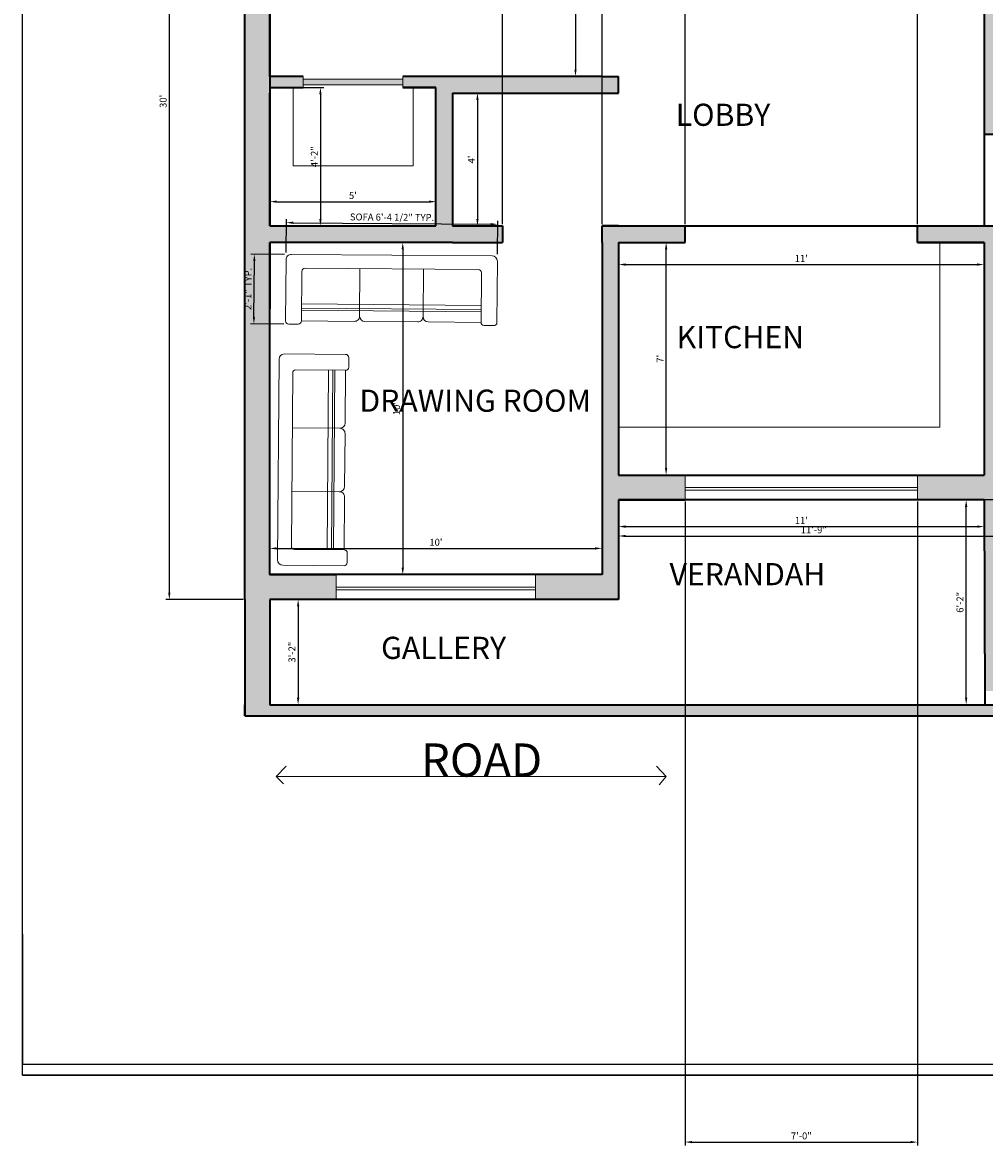
# Model space of a CAD drawing. Units: inches. Extents: x 2341 to 2872, y 1788 to 2419.
# Tile 1 of 3: x 2341 to 2689, y 1788 to 2194. Entities that reach past the tile are written whole.
import ezdxf

# ---------------------------------------------------------------- set-up
doc = ezdxf.new("R2010")
doc.units = ezdxf.units.IN
for name, color, linetype, lineweight in [('A-ANNO-DIMS', 2, 'Continuous', 18), ('A-ANNO-SYMB', 7, 'Continuous', 18), ('A-ANNO-TEXT', 7, 'Continuous', 25), ('A-ANNO-TTLB', 7, 'Continuous', 25), ('A-AREA-IDEN', 7, 'Continuous', 25), ('A-FLOR-FIXT', 9, 'Continuous', 18), ('A-FURN', 8, 'Continuous', 18), ('A-GLAZ', 4, 'Continuous', 18), ('A-WALL', 7, 'Continuous', 35)]:
    doc.layers.add(name, color=color, linetype=linetype, lineweight=lineweight)
doc.layers.add('A-WALL-PATT', color=18, linetype='Continuous', lineweight=13, true_color=0x000000)
doc.styles.get("Standard").update_dxf_attribs({"font": 'arial.ttf'})
doc.dimstyles.new('Copy of ISO-25', dxfattribs={"dimtxt": 2.5, "dimasz": 2.5, "dimexe": 1.25, "dimexo": 0.625, "dimtad": 1, "dimdec": 1, "dimlunit": 4, "dimtxsty": 'Standard', "dimcen": 2.5, "dimadec": 0, "dimazin": 0, "dimtfac": 1, "dimtdec": 1, "dimtmove": 0, "dimatfit": 3, "dimfxl": 1, "dimarcsym": 0})

# ---------------------------------------------------------------- blocks, each defined once
blk = doc.blocks.new('A$C05BA3A2B')
for p, q in [((0.05, 0.66), (1.95, 0.66)), ((0.05, 0.66), (1.95, 0.66)), ((0.05, 0.66), (1.95, 0.66)), ((0, 0.03), (0, 0.61)), ((0, 0.03), (0, 0.61)), ((0, 0.03), (0, 0.61)), ((2, 0.61), (2, 0.03)), ((2, 0.61), (2, 0.03)), ((2, 0.61), (2, 0.03)), ((0.15, 0.5), (0.15, 0.03)), ((0.15, 0.5), (0.15, 0.03)), ((0.15, 0.5), (0.15, 0.03)), ((1.82, 0.53), (0.18, 0.53)), ((1.82, 0.53), (0.18, 0.53)), ((1.82, 0.53), (0.18, 0.53)), ((0.7, 0.08), (0.7, 0.53)), ((0.7, 0.08), (0.7, 0.53)), ((0.7, 0.08), (0.7, 0.53)), ((1.3, 0.53), (1.3, 0.08)), ((1.3, 0.53), (1.3, 0.08)), ((1.3, 0.53), (1.3, 0.08)), ((1.85, 0.03), (1.85, 0.5)), ((1.85, 0.03), (1.85, 0.5)), ((1.85, 0.03), (1.85, 0.5)), ((1.85, 0.191), (0.15, 0.191)), ((1.85, 0.191), (0.15, 0.191)), ((1.85, 0.191), (0.15, 0.191)), ((1.85, 0.151), (0.15, 0.151)), ((1.85, 0.151), (0.15, 0.151)), ((1.85, 0.151), (0.15, 0.151)), ((1.85, 0.131), (0.15, 0.131)), ((1.85, 0.131), (0.15, 0.131)), ((1.85, 0.131), (0.15, 0.131)), ((0.12, 0), (0.03, 0)), ((0.12, 0), (0.03, 0)), ((0.12, 0), (0.03, 0)), ((0.65, 0.03), (0.15, 0.03)), ((0.65, 0.03), (0.15, 0.03)), ((0.65, 0.03), (0.15, 0.03)), ((1.25, 0.03), (0.75, 0.03)), ((1.25, 0.03), (0.75, 0.03)), ((1.25, 0.03), (0.75, 0.03)), ((1.85, 0.03), (1.35, 0.03)), ((1.85, 0.03), (1.35, 0.03)), ((1.85, 0.03), (1.35, 0.03)), ((1.97, 0), (1.88, 0)), ((1.97, 0), (1.88, 0)), ((1.97, 0), (1.88, 0))]:
    blk.add_line(p, q)
for centre, radius, start, end in [((0.05, 0.61), 0.05, 90, 180), ((0.05, 0.61), 0.05, 90, 180), ((0.05, 0.61), 0.05, 90, 180), ((1.95, 0.61), 0.05, 0, 90), ((1.95, 0.61), 0.05, 0, 90), ((1.95, 0.61), 0.05, 0, 90), ((0.18, 0.5), 0.03, 90, 180), ((0.18, 0.5), 0.03, 90, 180), ((0.18, 0.5), 0.03, 90, 180), ((1.82, 0.5), 0.03, 0, 90), ((1.82, 0.5), 0.03, 0, 90), ((1.82, 0.5), 0.03, 0, 90), ((0.03, 0.03), 0.03, 180, 270), ((0.03, 0.03), 0.03, 180, 270), ((0.03, 0.03), 0.03, 180, 270), ((0.12, 0.03), 0.03, 270, 0), ((0.12, 0.03), 0.03, 270, 0), ((0.12, 0.03), 0.03, 270, 0), ((0.65, 0.08), 0.05, 270, 0), ((0.65, 0.08), 0.05, 270, 0), ((0.65, 0.08), 0.05, 270, 0), ((0.75, 0.08), 0.05, 180, 270), ((0.75, 0.08), 0.05, 180, 270), ((0.75, 0.08), 0.05, 180, 270), ((1.25, 0.08), 0.05, 270, 0), ((1.25, 0.08), 0.05, 270, 0), ((1.25, 0.08), 0.05, 270, 0), ((1.35, 0.08), 0.05, 180, 270), ((1.35, 0.08), 0.05, 180, 270), ((1.35, 0.08), 0.05, 180, 270), ((1.88, 0.03), 0.03, 180, 270), ((1.88, 0.03), 0.03, 180, 270), ((1.88, 0.03), 0.03, 180, 270), ((1.97, 0.03), 0.03, 270, 0), ((1.97, 0.03), 0.03, 270, 0), ((1.97, 0.03), 0.03, 270, 0)]:
    blk.add_arc(centre, radius, start, end)
blk = doc.blocks.new('*D4')
at = {"layer": 'A-ANNO-DIMS', "color": 0, "lineweight": -2, "transparency": 16777216}
for p, q in [((2420.93, 2345.02), (2392.99, 2345.02)), ((2394.24, 2342.52), (2394.24, 1987.52)), ((2420.93, 1985.02), (2392.99, 1985.02))]:
    blk.add_line(p, q, dxfattribs=at)
at = {"layer": 'A-ANNO-DIMS', "color": 0, "transparency": 16777216}
for points in [[(2393.82, 2342.52), (2394.66, 2342.52), (2394.24, 2345.02)], [(2393.82, 1987.52), (2394.66, 1987.52), (2394.24, 1985.02)]]:
    blk.add_solid(points, dxfattribs=at)
at = {"layer": 'Defpoints', "color": 0, "transparency": 16777216}
for p in [(2421.55, 2345.02), (2394.24, 1985.02), (2421.55, 1985.02)]:
    blk.add_point(p, dxfattribs=at)
at = {"layer": 'A-ANNO-DIMS', "color": 0, "transparency": 16777216, "insert": (2392.34, 2165.02), "char_height": 2.5, "attachment_point": 5, "rotation": 90}
blk.add_mtext("30'", dxfattribs=at)
blk = doc.blocks.new('*D8')
at = {"layer": 'A-ANNO-DIMS', "color": 0, "lineweight": -2, "transparency": 16777216}
for p, q in [((2549.93, 2336.02), (2539.72, 2336.02)), ((2540.97, 2333.52), (2540.97, 2176.52)), ((2549.93, 2174.02), (2539.72, 2174.02))]:
    blk.add_line(p, q, dxfattribs=at)
at = {"layer": 'A-ANNO-DIMS', "color": 0, "transparency": 16777216}
for points in [[(2540.56, 2333.52), (2541.39, 2333.52), (2540.97, 2336.02)], [(2540.56, 2176.52), (2541.39, 2176.52), (2540.97, 2174.02)]]:
    blk.add_solid(points, dxfattribs=at)
at = {"layer": 'Defpoints', "color": 0, "transparency": 16777216}
for p in [(2550.55, 2336.02), (2540.97, 2174.02), (2550.55, 2174.02)]:
    blk.add_point(p, dxfattribs=at)
at = {"layer": 'A-ANNO-DIMS', "color": 0, "transparency": 16777216, "insert": (2539.07, 2255.02), "char_height": 2.5, "attachment_point": 5, "rotation": 90}
blk.add_mtext('13\'-6"', dxfattribs=at)
blk = doc.blocks.new('*D17')
at = {"layer": 'A-ANNO-DIMS', "color": 0, "lineweight": -2, "transparency": 16777216}
for p, q in [((2431.18, 2114.02), (2479.82, 2114.02)), ((2478.57, 2111.52), (2478.57, 1996.52)), ((2431.18, 1994.02), (2479.82, 1994.02))]:
    blk.add_line(p, q, dxfattribs=at)
at = {"layer": 'A-ANNO-DIMS', "color": 0, "transparency": 16777216}
for points in [[(2478.15, 2111.52), (2478.99, 2111.52), (2478.57, 2114.02)], [(2478.15, 1996.52), (2478.99, 1996.52), (2478.57, 1994.02)]]:
    blk.add_solid(points, dxfattribs=at)
at = {"layer": 'Defpoints', "color": 0, "transparency": 16777216}
for p in [(2430.55, 2114.02), (2430.55, 1994.02), (2478.57, 1994.02)]:
    blk.add_point(p, dxfattribs=at)
at = {"layer": 'A-ANNO-DIMS', "color": 0, "transparency": 16777216, "insert": (2476.67, 2054.02), "char_height": 2.5, "attachment_point": 5, "rotation": 90}
blk.add_mtext("10'", dxfattribs=at)
blk = doc.blocks.new('*D18')
at = {"layer": 'A-ANNO-DIMS', "color": 0, "lineweight": -2, "transparency": 16777216}
for p, q in [((2430.55, 1994.64), (2430.55, 2004.75)), ((2550.55, 1994.64), (2550.55, 2004.75)), ((2433.05, 2003.5), (2548.05, 2003.5))]:
    blk.add_line(p, q, dxfattribs=at)
at = {"layer": 'A-ANNO-DIMS', "color": 0, "transparency": 16777216}
for points in [[(2433.05, 2003.91), (2433.05, 2003.08), (2430.55, 2003.5)], [(2548.05, 2003.91), (2548.05, 2003.08), (2550.55, 2003.5)]]:
    blk.add_solid(points, dxfattribs=at)
at = {"layer": 'Defpoints', "color": 0, "transparency": 16777216}
for p in [(2550.55, 2003.5), (2430.55, 1994.02), (2550.55, 1994.02)]:
    blk.add_point(p, dxfattribs=at)
at = {"layer": 'A-ANNO-DIMS', "color": 0, "transparency": 16777216, "insert": (2490.55, 2005.4), "char_height": 2.5, "attachment_point": 5}
blk.add_mtext("10'", dxfattribs=at)
blk = doc.blocks.new('*D19')
at = {"layer": 'A-ANNO-DIMS', "color": 0, "lineweight": -2, "transparency": 16777216}
for p, q in [((2556.55, 2113.39), (2556.55, 2104.81)), ((2688.55, 2113.39), (2688.55, 2104.81)), ((2559.05, 2106.06), (2686.05, 2106.06))]:
    blk.add_line(p, q, dxfattribs=at)
at = {"layer": 'A-ANNO-DIMS', "color": 0, "transparency": 16777216}
for points in [[(2559.05, 2106.47), (2559.05, 2105.64), (2556.55, 2106.06)], [(2686.05, 2106.47), (2686.05, 2105.64), (2688.55, 2106.06)]]:
    blk.add_solid(points, dxfattribs=at)
at = {"layer": 'Defpoints', "color": 0, "transparency": 16777216}
for p in [(2556.55, 2114.02), (2688.55, 2114.02), (2688.55, 2106.06)]:
    blk.add_point(p, dxfattribs=at)
at = {"layer": 'A-ANNO-DIMS', "color": 0, "transparency": 16777216, "insert": (2622.55, 2107.94), "char_height": 2.5, "attachment_point": 5}
blk.add_mtext("11'", dxfattribs=at)
blk = doc.blocks.new('*D20')
at = {"layer": 'A-ANNO-DIMS', "color": 0, "lineweight": -2, "transparency": 16777216}
for p, q in [((2557.18, 2114.02), (2574.96, 2114.02)), ((2573.71, 2032.52), (2573.71, 2111.52)), ((2557.18, 2030.02), (2574.96, 2030.02))]:
    blk.add_line(p, q, dxfattribs=at)
at = {"layer": 'A-ANNO-DIMS', "color": 0, "transparency": 16777216}
for points in [[(2573.3, 2111.52), (2574.13, 2111.52), (2573.71, 2114.02)], [(2573.3, 2032.52), (2574.13, 2032.52), (2573.71, 2030.02)]]:
    blk.add_solid(points, dxfattribs=at)
at = {"layer": 'Defpoints', "color": 0, "transparency": 16777216}
for p in [(2556.55, 2114.02), (2573.71, 2114.02), (2556.55, 2030.02)]:
    blk.add_point(p, dxfattribs=at)
at = {"layer": 'A-ANNO-DIMS', "color": 0, "transparency": 16777216, "insert": (2571.84, 2072.02), "char_height": 2.5, "attachment_point": 5, "rotation": 90}
blk.add_mtext("7'", dxfattribs=at)
blk = doc.blocks.new('*D21')
at = {"layer": 'A-ANNO-DIMS', "color": 0, "lineweight": -2, "transparency": 16777216}
for p, q in [((2556.55, 2020.39), (2556.55, 2006.73)), ((2697.55, 2020.39), (2697.55, 2006.73)), ((2559.05, 2007.98), (2695.05, 2007.98))]:
    blk.add_line(p, q, dxfattribs=at)
at = {"layer": 'A-ANNO-DIMS', "color": 0, "transparency": 16777216}
for points in [[(2559.05, 2008.4), (2559.05, 2007.57), (2556.55, 2007.98)], [(2695.05, 2008.4), (2695.05, 2007.57), (2697.55, 2007.98)]]:
    blk.add_solid(points, dxfattribs=at)
at = {"layer": 'Defpoints', "color": 0, "transparency": 16777216}
for p in [(2556.55, 2021.02), (2697.55, 2021.02), (2697.55, 2007.98)]:
    blk.add_point(p, dxfattribs=at)
at = {"layer": 'A-ANNO-DIMS', "color": 0, "transparency": 16777216, "insert": (2627.05, 2009.89), "char_height": 2.5, "attachment_point": 5}
blk.add_mtext('11\'-9"', dxfattribs=at)
blk = doc.blocks.new('*D22')
at = {"layer": 'A-ANNO-DIMS', "color": 0, "lineweight": -2, "transparency": 16777216}
for p, q in [((2696.93, 2021.02), (2680.85, 2021.02)), ((2682.1, 1949.52), (2682.1, 2018.52)), ((2696.93, 1947.02), (2680.85, 1947.02))]:
    blk.add_line(p, q, dxfattribs=at)
at = {"layer": 'A-ANNO-DIMS', "color": 0, "transparency": 16777216}
for points in [[(2681.68, 2018.52), (2682.52, 2018.52), (2682.1, 2021.02)], [(2681.68, 1949.52), (2682.52, 1949.52), (2682.1, 1947.02)]]:
    blk.add_solid(points, dxfattribs=at)
at = {"layer": 'Defpoints', "color": 0, "transparency": 16777216}
for p in [(2682.1, 2021.02), (2697.55, 2021.02), (2697.55, 1947.02)]:
    blk.add_point(p, dxfattribs=at)
at = {"layer": 'A-ANNO-DIMS', "color": 0, "transparency": 16777216, "insert": (2680.2, 1984.02), "char_height": 2.5, "attachment_point": 5, "rotation": 90}
blk.add_mtext('6\'-2"', dxfattribs=at)
blk = doc.blocks.new('*D23')
at = {"layer": 'A-ANNO-DIMS', "color": 0, "lineweight": -2, "transparency": 16777216}
for p, q in [((2431.18, 1985.02), (2442.02, 1985.02)), ((2440.77, 1982.52), (2440.77, 1949.52)), ((2431.18, 1947.02), (2442.02, 1947.02))]:
    blk.add_line(p, q, dxfattribs=at)
at = {"layer": 'A-ANNO-DIMS', "color": 0, "transparency": 16777216}
for points in [[(2440.35, 1982.52), (2441.19, 1982.52), (2440.77, 1985.02)], [(2440.35, 1949.52), (2441.19, 1949.52), (2440.77, 1947.02)]]:
    blk.add_solid(points, dxfattribs=at)
at = {"layer": 'Defpoints', "color": 0, "transparency": 16777216}
for p in [(2430.55, 1985.02), (2430.55, 1947.02), (2440.77, 1947.02)]:
    blk.add_point(p, dxfattribs=at)
at = {"layer": 'A-ANNO-DIMS', "color": 0, "transparency": 16777216, "insert": (2438.87, 1966.02), "char_height": 2.5, "attachment_point": 5, "rotation": 90}
blk.add_mtext('3\'-2"', dxfattribs=at)
blk = doc.blocks.new('*D24')
at = {"layer": 'A-ANNO-DIMS', "color": 0, "lineweight": -2, "transparency": 16777216}
for p, q in [((2430.55, 2120.64), (2430.55, 2130.02)), ((2433.05, 2128.77), (2488.05, 2128.77)), ((2490.55, 2120.64), (2490.55, 2130.02))]:
    blk.add_line(p, q, dxfattribs=at)
at = {"layer": 'A-ANNO-DIMS', "color": 0, "transparency": 16777216}
for points in [[(2433.05, 2129.19), (2433.05, 2128.36), (2430.55, 2128.77)], [(2488.05, 2129.19), (2488.05, 2128.36), (2490.55, 2128.77)]]:
    blk.add_solid(points, dxfattribs=at)
at = {"layer": 'Defpoints', "color": 0, "transparency": 16777216}
for p in [(2490.55, 2128.77), (2430.55, 2120.02), (2490.55, 2120.02)]:
    blk.add_point(p, dxfattribs=at)
at = {"layer": 'A-ANNO-DIMS', "color": 0, "transparency": 16777216, "insert": (2460.55, 2130.67), "char_height": 2.5, "attachment_point": 5}
blk.add_mtext("5'", dxfattribs=at)
blk = doc.blocks.new('*D25')
at = {"layer": 'A-ANNO-DIMS', "color": 0, "lineweight": -2, "transparency": 16777216}
for p, q in [((2431.18, 2170.02), (2450.08, 2170.02)), ((2448.83, 2167.52), (2448.83, 2122.52)), ((2431.18, 2120.02), (2450.08, 2120.02))]:
    blk.add_line(p, q, dxfattribs=at)
at = {"layer": 'A-ANNO-DIMS', "color": 0, "transparency": 16777216}
for points in [[(2448.41, 2167.52), (2449.25, 2167.52), (2448.83, 2170.02)], [(2448.41, 2122.52), (2449.25, 2122.52), (2448.83, 2120.02)]]:
    blk.add_solid(points, dxfattribs=at)
at = {"layer": 'Defpoints', "color": 0, "transparency": 16777216}
for p in [(2430.55, 2170.02), (2430.55, 2120.02), (2448.83, 2120.02)]:
    blk.add_point(p, dxfattribs=at)
at = {"layer": 'A-ANNO-DIMS', "color": 0, "transparency": 16777216, "insert": (2446.95, 2145.02), "char_height": 2.5, "attachment_point": 5, "rotation": 90}
blk.add_mtext('4\'-2"', dxfattribs=at)
blk = doc.blocks.new('*D26')
at = {"layer": 'A-ANNO-DIMS', "color": 0, "lineweight": -2, "transparency": 16777216}
for p, q in [((2556.55, 2020.39), (2556.55, 2010.13)), ((2688.59, 2020.39), (2688.59, 2010.13)), ((2559.05, 2011.38), (2686.09, 2011.38))]:
    blk.add_line(p, q, dxfattribs=at)
at = {"layer": 'A-ANNO-DIMS', "color": 0, "transparency": 16777216}
for points in [[(2559.05, 2011.8), (2559.05, 2010.97), (2556.55, 2011.38)], [(2686.09, 2011.8), (2686.09, 2010.97), (2688.59, 2011.38)]]:
    blk.add_solid(points, dxfattribs=at)
at = {"layer": 'Defpoints', "color": 0, "transparency": 16777216}
for p in [(2556.55, 2021.02), (2688.59, 2021.02), (2688.59, 2011.38)]:
    blk.add_point(p, dxfattribs=at)
at = {"layer": 'A-ANNO-DIMS', "color": 0, "transparency": 16777216, "insert": (2622.57, 2013.26), "char_height": 2.5, "attachment_point": 5}
blk.add_mtext("11'", dxfattribs=at)
blk = doc.blocks.new('*D30')
at = {"layer": 'A-ANNO-DIMS', "color": 0, "lineweight": -2, "transparency": 16777216}
for p, q in [((2497.18, 2168.02), (2506.8, 2168.02)), ((2505.55, 2165.52), (2505.55, 2122.52)), ((2497.18, 2120.02), (2506.8, 2120.02))]:
    blk.add_line(p, q, dxfattribs=at)
at = {"layer": 'A-ANNO-DIMS', "color": 0, "transparency": 16777216}
for points in [[(2505.14, 2165.52), (2505.97, 2165.52), (2505.55, 2168.02)], [(2505.14, 2122.52), (2505.97, 2122.52), (2505.55, 2120.02)]]:
    blk.add_solid(points, dxfattribs=at)
at = {"layer": 'Defpoints', "color": 0, "transparency": 16777216}
for p in [(2496.55, 2168.02), (2496.55, 2120.02), (2505.55, 2120.02)]:
    blk.add_point(p, dxfattribs=at)
at = {"layer": 'A-ANNO-DIMS', "color": 0, "transparency": 16777216, "insert": (2503.68, 2144.02), "char_height": 2.5, "attachment_point": 5, "rotation": 90}
blk.add_mtext("4'", dxfattribs=at)
blk = doc.blocks.new('*D33')
at = {"layer": 'A-ANNO-DIMS', "color": 0, "lineweight": -2, "transparency": 16777216}
for p, q in [((2436.43, 2110.36), (2436.52, 2122.44)), ((2439.01, 2121.17), (2510.35, 2120.63)), ((2512.77, 2109.78), (2512.86, 2121.86))]:
    blk.add_line(p, q, dxfattribs=at)
at = {"layer": 'A-ANNO-DIMS', "color": 0, "transparency": 16777216}
for points in [[(2439.02, 2121.58), (2439.01, 2120.75), (2436.51, 2121.19)], [(2510.36, 2121.04), (2510.35, 2120.21), (2512.85, 2120.61)]]:
    blk.add_solid(points, dxfattribs=at)
at = {"layer": 'Defpoints', "color": 0, "transparency": 16777216}
for p in [(2512.85, 2120.61), (2436.43, 2109.73), (2512.77, 2109.16)]:
    blk.add_point(p, dxfattribs=at)
at = {"layer": 'A-ANNO-DIMS', "color": 0, "transparency": 16777216, "insert": (2474.7, 2122.82), "char_height": 2.5, "attachment_point": 5, "rotation": 359.5672}
blk.add_mtext('SOFA 6\'-4 1/2" TYP.', dxfattribs=at)
blk = doc.blocks.new('*D34')
at = {"layer": 'A-ANNO-DIMS', "color": 0, "lineweight": -2, "transparency": 16777216}
for p, q in [((2435.8, 2109.74), (2423.73, 2109.83)), ((2424.8, 2087.14), (2424.96, 2107.32)), ((2435.61, 2084.56), (2423.54, 2084.65))]:
    blk.add_line(p, q, dxfattribs=at)
at = {"layer": 'A-ANNO-DIMS', "color": 0, "transparency": 16777216}
for points in [[(2424.54, 2107.32), (2425.37, 2107.32), (2424.98, 2109.82)], [(2424.39, 2087.15), (2425.22, 2087.14), (2424.79, 2084.64)]]:
    blk.add_solid(points, dxfattribs=at)
at = {"layer": 'Defpoints', "color": 0, "transparency": 16777216}
for p in [(2424.98, 2109.82), (2436.43, 2109.73), (2436.24, 2084.56)]:
    blk.add_point(p, dxfattribs=at)
at = {"layer": 'A-ANNO-DIMS', "color": 0, "transparency": 16777216, "insert": (2423, 2097.25), "char_height": 2.5, "attachment_point": 5, "rotation": 89.5672}
blk.add_mtext('2\'-1" TYP.', dxfattribs=at)
blk = doc.blocks.new('*D36')
at = {"layer": 'A-ANNO-DIMS', "color": 0, "lineweight": -2, "transparency": 16777216}
for p, q in [((2580.55, 2020.39), (2580.55, 1787.77)), ((2664.55, 2020.39), (2664.55, 1787.77)), ((2583.05, 1789.02), (2662.05, 1789.02))]:
    blk.add_line(p, q, dxfattribs=at)
at = {"layer": 'A-ANNO-DIMS', "color": 0, "transparency": 16777216}
for points in [[(2583.05, 1789.43), (2583.05, 1788.6), (2580.55, 1789.02)], [(2662.05, 1789.43), (2662.05, 1788.6), (2664.55, 1789.02)]]:
    blk.add_solid(points, dxfattribs=at)
at = {"layer": 'Defpoints', "color": 0, "transparency": 16777216}
for p in [(2580.55, 2021.02), (2664.55, 2021.02), (2664.55, 1789.02)]:
    blk.add_point(p, dxfattribs=at)
at = {"layer": 'A-ANNO-DIMS', "color": 0, "transparency": 16777216, "insert": (2622.55, 1790.92), "char_height": 2.5, "attachment_point": 5}
blk.add_mtext('7\'-0"', dxfattribs=at)
blk = doc.blocks.new('*D37')
at = {"layer": 'A-ANNO-DIMS', "color": 0, "lineweight": -2, "transparency": 16777216}
for p, q in [((2580.55, 2120.64), (2580.55, 2374.42)), ((2664.55, 2120.64), (2664.55, 2374.42)), ((2583.05, 2373.17), (2662.05, 2373.17))]:
    blk.add_line(p, q, dxfattribs=at)
at = {"layer": 'A-ANNO-DIMS', "color": 0, "transparency": 16777216}
for points in [[(2583.05, 2373.58), (2583.05, 2372.75), (2580.55, 2373.17)], [(2662.05, 2373.58), (2662.05, 2372.75), (2664.55, 2373.17)]]:
    blk.add_solid(points, dxfattribs=at)
at = {"layer": 'Defpoints', "color": 0, "transparency": 16777216}
for p in [(2664.55, 2373.17), (2580.55, 2120.02), (2664.55, 2120.02)]:
    blk.add_point(p, dxfattribs=at)
at = {"layer": 'A-ANNO-DIMS', "color": 0, "transparency": 16777216, "insert": (2622.55, 2375.07), "char_height": 2.5, "attachment_point": 5}
blk.add_mtext('7\'-0"', dxfattribs=at)
blk = doc.blocks.new('*D38')
at = {"layer": 'A-ANNO-DIMS', "color": 0, "lineweight": -2, "transparency": 16777216}
for p, q in [((2514.55, 2120.64), (2514.55, 2374.42)), ((2550.55, 2120.64), (2550.55, 2374.42)), ((2517.05, 2373.17), (2548.05, 2373.17))]:
    blk.add_line(p, q, dxfattribs=at)
at = {"layer": 'A-ANNO-DIMS', "color": 0, "transparency": 16777216}
for points in [[(2517.05, 2373.58), (2517.05, 2372.75), (2514.55, 2373.17)], [(2548.05, 2373.58), (2548.05, 2372.75), (2550.55, 2373.17)]]:
    blk.add_solid(points, dxfattribs=at)
at = {"layer": 'Defpoints', "color": 0, "transparency": 16777216}
for p in [(2550.55, 2373.17), (2514.55, 2120.02), (2550.55, 2120.02)]:
    blk.add_point(p, dxfattribs=at)
at = {"layer": 'A-ANNO-DIMS', "color": 0, "transparency": 16777216, "insert": (2532.55, 2375.07), "char_height": 2.5, "attachment_point": 5}
blk.add_mtext('3\'-0"', dxfattribs=at)

msp = doc.modelspace()

# ---------------------------------------------------------------- hatches: boundary and pattern name
at = {"layer": 'A-WALL-PATT'}
h = msp.add_hatch(color=256, dxfattribs=at)
h.dxf.hatch_style = 1
h.paths.add_polyline_path([(2781.55, 2345.02), (2421.55, 2345.02), (2421.55, 1985.02), (2421.55, 1949.02), (2421.55, 1943.02), (2781.55, 1943.02), (2781.55, 1985.02)])
h.paths.add_polyline_path([(2550.55, 2336.02), (2772.55, 2336.02), (2772.55, 1994.02), (2772.55, 1985.02), (2772.55, 1947.02), (2430.55, 1947.02), (2430.55, 1985.02), (2454.55, 1985.02), (2454.55, 1994.02), (2430.55, 1994.02), (2430.55, 2114.02), (2496.55, 2114.02), (2514.55, 2114.02), (2514.55, 2120.02), (2496.55, 2120.02), (2496.55, 2168.02), (2556.55, 2168.02), (2556.55, 2174.02), (2550.55, 2174.02), (2478.55, 2174.02), (2478.55, 2170.02), (2490.55, 2170.02), (2490.55, 2168.02), (2490.55, 2120.02), (2430.55, 2120.02), (2430.55, 2168.02), (2430.55, 2174.02), (2430.55, 2204.02), (2430.55, 2336.02)], flags=16)
h.paths.add_polyline_path([(2556.55, 2336.02), (2652.55, 2336.02), (2652.55, 2198.02), (2646.55, 2198.02), (2601.55, 2198.02), (2595.55, 2198.02), (2595.55, 2240.02), (2556.55, 2240.02), (2556.55, 2246.02), (2556.55, 2294.02)], flags=0)
h.paths.add_polyline_path([(2556.55, 2300.02), (2646.55, 2300.02), (2646.55, 2294.02), (2646.55, 2204.02), (2601.55, 2204.02), (2601.55, 2246.02), (2601.55, 2294.02), (2613.55, 2294.02), (2613.55, 2300.02), (2592.55, 2300.02), (2592.55, 2294.02), (2595.55, 2294.02), (2595.55, 2246.02), (2556.55, 2246.02), (2556.55, 2282.02)], flags=0)
h.paths.add_polyline_path([(2680.26, 2307.06), (2747.77, 2307.06), (2747.77, 2329.57), (2770.28, 2329.57), (2770.28, 2307.06), (2770.28, 2239.54), (2770.28, 2217.04), (2747.77, 2217.04), (2747.77, 2239.54), (2680.26, 2239.54)], flags=0)
h.paths.add_polyline_path([(2681.16, 2306.16), (2769.38, 2306.16), (2769.38, 2240.44), (2704.56, 2240.44, -0.009128), (2703.54, 2240.44), (2681.16, 2240.44)], flags=0)
h.paths.add_polyline_path([(2744.14, 2298.19), (2744.14, 2293.47), (2696.44, 2293.47), (2696.44, 2242.73, -0.092104), (2691.71, 2247), (2691.71, 2298.19)], flags=0)
h.paths.add_polyline_path([(2694.86, 2296.62), (2694.86, 2295.04), (2693.29, 2295.04), (2693.29, 2296.62)], flags=0)
h.paths.add_polyline_path([(2478.55, 2173.02), (2478.55, 2172.02), (2478.55, 2171.02), (2442.55, 2171.02), (2442.55, 2170.02), (2438.98, 2170.02), (2430.55, 2170.02), (2430.55, 2174.02), (2442.55, 2174.02), (2442.55, 2173.02)], flags=0)
h.paths.add_polyline_path([(2688.55, 2198.02), (2697.55, 2198.02), (2772.55, 2198.02), (2772.55, 2189.02), (2772.55, 2153.02), (2755.26, 2153.02), (2755.26, 2145.02), (2772.55, 2145.02), (2772.55, 2137.02), (2755.26, 2137.02), (2755.26, 2129.02), (2772.55, 2129.02), (2772.55, 2121.02), (2755.26, 2121.02), (2755.26, 2119.07), (2757.66, 2119.07), (2755.26, 2113.02), (2772.55, 2113.02), (2772.55, 2105.02), (2736.55, 2105.02), (2736.55, 2153.02), (2697.55, 2153.02), (2697.55, 2021.02), (2697.55, 1952.02), (2688.89, 1952.02), (2688.89, 1947.02), (2688.59, 2021.02), (2688.55, 2021.02), (2580.55, 2021.02), (2580.55, 2030.02), (2556.55, 2030.02), (2556.55, 2114.02), (2580.55, 2114.02), (2580.55, 2120.02), (2664.55, 2120.02), (2688.55, 2120.02), (2688.55, 2189.02)], flags=0)
h.paths.add_polyline_path([(2510.86, 2109.17, -0.414214), (2512.75, 2107.25), (2512.59, 2085.13, -0.414214), (2511.43, 2083.99), (2508, 2084.02, -0.414214), (2506.86, 2085.17), (2487.78, 2085.31, -0.414214), (2485.88, 2087.24, -0.414214), (2483.96, 2085.34), (2464.87, 2085.49, -0.414214), (2462.98, 2087.41, -0.414214), (2461.06, 2085.52), (2441.97, 2085.66, -0.414214), (2440.82, 2084.52), (2437.38, 2084.55, -0.414214), (2436.25, 2085.7), (2436.41, 2107.83, -0.414214), (2438.34, 2109.72)], flags=0)
h.paths.add_polyline_path([(2736.55, 2189.02), (2736.55, 2170), (2728.55, 2170), (2728.55, 2153.02), (2720.55, 2153.02), (2720.55, 2189.02), (2712.55, 2189.02), (2712.55, 2153.02), (2704.55, 2153.02), (2704.55, 2189.02)], flags=0)
edge = h.paths.add_edge_path(flags=0)
edge.add_ellipse((2759.52, 2317.47), major_axis=(6.08, 0), ratio=0.975448, start_angle=450, end_angle=540, ccw=False)
edge.add_ellipse((2759.52, 2317.47), major_axis=(6.08, 0), ratio=0.975448, start_angle=360, end_angle=450, ccw=False)
edge.add_ellipse((2759.52, 2317.47), major_axis=(6.08, 0), ratio=0.975448, start_angle=270, end_angle=360, ccw=False)
edge.add_ellipse((2759.52, 2317.47), major_axis=(6.08, 0), ratio=0.975448, start_angle=180, end_angle=270, ccw=False)
h.paths.add_polyline_path([(2505.86, 2104.26, -0.414214), (2507, 2103.11), (2506.89, 2089.02), (2442, 2089.51), (2442.11, 2103.6, -0.414214), (2443.26, 2104.74)], flags=0)
h.paths.add_polyline_path([(2485.9, 2089.94), (2463, 2090.11), (2463.01, 2091.64), (2485.91, 2091.47)], flags=0)
h.paths.add_polyline_path([(2758.23, 2298.35), (2764.61, 2298.35, -0.414214), (2768.21, 2294.75), (2768.21, 2280.47, -0.414214), (2764.61, 2276.87), (2758.23, 2276.87, -0.414214), (2754.62, 2280.47), (2754.62, 2294.75, -0.414214)], flags=0)
h.paths.add_polyline_path([(2758.23, 2297.45), (2764.61, 2297.45, -0.414214), (2767.31, 2294.75), (2767.31, 2280.47, -0.414214), (2764.61, 2277.77), (2758.23, 2277.77, -0.414214), (2755.52, 2280.47), (2755.52, 2294.75, -0.414214)], flags=0)
h.paths.add_polyline_path([(2758.23, 2265.42), (2764.61, 2265.42, -0.414214), (2768.21, 2261.82), (2768.21, 2247.53, -0.414214), (2764.61, 2243.93), (2758.23, 2243.93, -0.414214), (2754.62, 2247.53), (2754.62, 2261.82, -0.414214)], flags=0)
h.paths.add_polyline_path([(2758.23, 2264.52), (2764.61, 2264.52, -0.414214), (2767.31, 2261.82), (2767.31, 2247.53, -0.414214), (2764.61, 2244.83), (2758.23, 2244.83, -0.414214), (2755.52, 2247.53), (2755.52, 2261.82, -0.414214)], flags=0)
edge = h.paths.add_edge_path(flags=0)
edge.add_ellipse((2759.52, 2229.13), major_axis=(6.08, 0), ratio=0.975448, start_angle=90, end_angle=180, ccw=False)
edge.add_ellipse((2759.52, 2229.13), major_axis=(6.08, 0), ratio=0.975448, start_angle=0, end_angle=90, ccw=False)
edge.add_ellipse((2759.52, 2229.13), major_axis=(6.08, 0), ratio=0.975448, start_angle=270, end_angle=360, ccw=False)
edge.add_ellipse((2759.52, 2229.13), major_axis=(6.08, 0), ratio=0.975448, start_angle=180, end_angle=270, ccw=False)
h.paths.add_polyline_path([(2457.94, 2073.59, -0.414214), (2459.08, 2072.44), (2459.05, 2069, -0.414214), (2457.9, 2067.87), (2457.75, 2048.78, -0.414214), (2455.83, 2046.89, -0.414214), (2457.72, 2044.96), (2457.58, 2025.88, -0.414214), (2455.66, 2023.98, -0.414214), (2457.55, 2022.06), (2457.41, 2002.98, -0.414214), (2458.54, 2001.82), (2458.52, 1998.39, -0.414214), (2457.36, 1997.25), (2435.24, 1997.42, -0.414214), (2433.35, 1999.34), (2433.89, 2071.86, -0.414214), (2435.82, 2073.76)], flags=0)
h.paths.add_polyline_path([(2454.05, 2067.89), (2453.56, 2003), (2439.47, 2003.11, -0.414214), (2438.33, 2004.26), (2438.8, 2066.86, -0.414214), (2439.96, 2068)], flags=0)
h.paths.add_polyline_path([(2452.95, 2024), (2451.43, 2024.02), (2451.6, 2046.92), (2453.13, 2046.91)], flags=0)
h.paths.add_polyline_path([(2830.4, 1819.46), (2838.99, 1819.46), (2838.99, 1828.46), (2830.4, 1828.46)], flags=9)
h.paths.add_polyline_path([(2814.93, 1841.19), (2823.62, 1841.19), (2823.62, 1850.5), (2814.93, 1850.5)], flags=9)
h.paths.add_polyline_path([(2843.19, 1840.36), (2852.25, 1840.36), (2852.25, 1849.36), (2843.19, 1849.36)], flags=9)
h.paths.add_polyline_path([(2828.19, 1854.15), (2839.1, 1854.15), (2839.1, 1863.15), (2828.19, 1863.15)], flags=9)
h.paths.add_polyline_path([(2760.12, 1830.89), (2792.1, 1830.89), (2792.1, 1840.21), (2760.12, 1840.21)], flags=9)
h.paths.add_polyline_path([(2760.12, 1840.53), (2800.48, 1840.53), (2800.48, 1849.85), (2760.12, 1849.85)], flags=9)
h.paths.add_polyline_path([(2758.73, 1854.24), (2815.82, 1854.24), (2815.82, 1863.56), (2758.73, 1863.56)], flags=9)
h.paths.add_polyline_path([(2482.08, 1917.73), (2536.72, 1917.73), (2536.72, 1936.36), (2482.08, 1936.36)], flags=9)
h.paths.add_polyline_path([(2707.72, 1951.32), (2770.13, 1951.32), (2770.13, 1963.73), (2707.72, 1963.73)], flags=8)
h.paths.add_polyline_path([(2706.05, 2121.97), (2725.65, 2121.97), (2725.65, 2134.17), (2706.05, 2134.17)], flags=8)
h.paths.add_polyline_path([(2705.12, 1972.11), (2749.62, 1972.11), (2749.62, 1984.52), (2705.12, 1984.52)], flags=8)
h.paths.add_polyline_path([(2468.66, 1961.36), (2524.36, 1961.36), (2524.36, 1973.77), (2468.66, 1973.77)], flags=8)
h.paths.add_polyline_path([(2572.95, 1988.2), (2639.05, 1988.2), (2639.05, 2000.2), (2572.95, 2000.2)], flags=8)
h.paths.add_polyline_path([(2460.85, 2050.66), (2556.87, 2050.66), (2556.87, 2063.08), (2460.85, 2063.08)], flags=8)
h.paths.add_polyline_path([(2575.44, 2073.64), (2628.63, 2073.64), (2628.63, 2086.04), (2575.44, 2086.04)], flags=8)
h.paths.add_polyline_path([(2575.12, 2153.95), (2616.53, 2153.95), (2616.53, 2166.37), (2575.12, 2166.37)], flags=8)
h.paths.add_polyline_path([(2664.33, 2218.95), (2729.32, 2218.95), (2729.32, 2231.37), (2664.33, 2231.37)], flags=8)
h.paths.add_polyline_path([(2557.77, 2265.61), (2586.74, 2265.61), (2586.74, 2278.02), (2557.77, 2278.02)], flags=8)
h.paths.add_polyline_path([(2605.48, 2263.57), (2639.29, 2263.57), (2639.29, 2275.57), (2605.48, 2275.57)], flags=8)
h.paths.add_polyline_path([(2569.54, 2309.66), (2602.87, 2309.66), (2602.87, 2322.07), (2569.54, 2322.07)], flags=8)
h.paths.add_polyline_path([(2458.16, 2214.67), (2523.15, 2214.67), (2523.15, 2227.09), (2458.16, 2227.09)], flags=8)
h.paths.add_polyline_path([(2458.16, 2227.52), (2511.98, 2227.52), (2511.98, 2239.93), (2458.16, 2239.93)], flags=8)
h.paths.add_polyline_path([(2449.57, 2140.97), (2449.57, 2149.18), (2444.42, 2149.18), (2444.42, 2140.97)], flags=8)
h.paths.add_polyline_path([(2458.63, 2128.07), (2462.49, 2128.07), (2462.49, 2133.23), (2458.63, 2133.23)], flags=8)
h.paths.add_polyline_path([(2506.29, 2142.15), (2506.29, 2146.01), (2501.14, 2146.01), (2501.14, 2142.15)], flags=8)
h.paths.add_polyline_path([(2487.54, 2002.8), (2493.34, 2002.8), (2493.34, 2007.95), (2487.54, 2007.95)], flags=8)
h.paths.add_polyline_path([(2479.27, 2051.01), (2479.27, 2056.81), (2474.12, 2056.81), (2474.12, 2051.01)], flags=8)
h.paths.add_polyline_path([(2441.47, 1961.92), (2441.47, 1970.13), (2436.31, 1970.13), (2436.31, 1961.92)], flags=8)
h.paths.add_polyline_path([(2682.8, 1979.93), (2682.8, 1988.13), (2677.65, 1988.13), (2677.65, 1979.93)], flags=8)
h.paths.add_polyline_path([(2752.63, 2088.44), (2756.49, 2088.44), (2756.49, 2093.6), (2752.63, 2093.6)], flags=8)
h.paths.add_polyline_path([(2752.63, 2180.4), (2756.49, 2180.4), (2756.49, 2185.55), (2752.63, 2185.55)], flags=8)
h.paths.add_polyline_path([(2740.86, 2261.83), (2740.86, 2271.98), (2735.71, 2271.98), (2735.71, 2261.83)], flags=8)
h.paths.add_polyline_path([(2709.54, 2328.87), (2715.34, 2328.87), (2715.34, 2334.02), (2709.54, 2334.02)], flags=8)
h.paths.add_polyline_path([(2639.95, 2316.1), (2639.95, 2319.95), (2634.8, 2319.95), (2634.8, 2316.1)], flags=8)
h.paths.add_polyline_path([(2597.45, 2328.64), (2605.65, 2328.64), (2605.65, 2333.8), (2597.45, 2333.8)], flags=8)
h.paths.add_polyline_path([(2487.54, 2325.01), (2493.34, 2325.01), (2493.34, 2330.16), (2487.54, 2330.16)], flags=8)
h.paths.add_polyline_path([(2541.67, 2249.83), (2541.67, 2259.98), (2536.52, 2259.98), (2536.52, 2249.83)], flags=8)
h = msp.add_hatch(color=256, dxfattribs=at)
h.dxf.hatch_style = 1
h.paths.add_polyline_path([(2556.55, 1994.02), (2556.55, 2021.02), (2580.55, 2021.02), (2580.55, 2030.02), (2556.55, 2030.02), (2556.55, 2114.02), (2580.55, 2114.02), (2580.55, 2120.02), (2556.55, 2120.02), (2550.55, 2120.02), (2550.55, 2114.02), (2550.55, 1994.02), (2526.55, 1994.02), (2526.55, 1985.02), (2556.55, 1985.02)])
h.paths.add_polyline_path([(2697.55, 2120.02), (2688.55, 2120.02), (2664.55, 2120.02), (2664.55, 2114.02), (2688.55, 2114.02), (2688.55, 2030.02), (2664.55, 2030.02), (2664.55, 2021.02), (2688.55, 2021.02), (2688.59, 2021.02), (2688.87, 1952.02), (2697.55, 1952.02), (2697.55, 2021.02)])
h.paths.add_polyline_path([(2772.55, 2198.02), (2688.55, 2198.02), (2688.55, 2189.02), (2688.55, 2153.02), (2697.55, 2153.02), (2697.55, 2189.02), (2772.55, 2189.02)])
h.paths.add_polyline_path([(2652.55, 2336.02), (2646.55, 2336.02), (2646.55, 2204.02), (2601.55, 2204.02), (2601.55, 2246.02), (2601.55, 2294.02), (2613.55, 2294.02), (2613.55, 2296.02), (2634.55, 2296.02), (2634.55, 2294.02), (2646.55, 2294.02), (2646.55, 2300.02), (2646.55, 2336.02), (2556.55, 2336.02), (2556.55, 2294.02), (2568.55, 2294.02), (2568.55, 2296.02), (2592.55, 2296.02), (2592.55, 2294.02), (2595.55, 2294.02), (2595.55, 2246.02), (2556.55, 2246.02), (2556.55, 2240.02), (2595.55, 2240.02), (2595.55, 2198.02), (2601.55, 2198.02), (2646.55, 2198.02), (2652.55, 2198.02)])
h.paths.add_polyline_path([(2442.55, 2174.02), (2430.55, 2174.02), (2430.55, 2170.02), (2442.55, 2170.02)])
h.paths.add_polyline_path([(2478.55, 2172.02), (2478.55, 2173.02), (2442.55, 2173.02), (2442.55, 2171.02), (2478.55, 2171.02)])
h.paths.add_polyline_path([(2556.55, 2336.02), (2550.55, 2336.02), (2550.55, 2210.02), (2556.55, 2210.02)])
h.paths.add_polyline_path([(2460.85, 2050.66), (2556.87, 2050.66), (2556.87, 2063.08), (2460.85, 2063.08)], flags=9)
h.paths.add_polyline_path([(2569.54, 2309.66), (2602.87, 2309.66), (2602.87, 2322.07), (2569.54, 2322.07)], flags=24)

# ---------------------------------------------------------------- linework, layer by layer
at = {"layer": 'A-ANNO-SYMB'}
for p, q in [((2432.82, 1921.04), (2436.49, 1924.77)), ((2573.7, 1921.04), (2570.21, 1924.77)), ((2485.19, 1921.04), (2432.82, 1921.04)), ((2432.82, 1921.04), (2435.46, 1918.44)), ((2485.19, 1921.04), (2573.7, 1921.04)), ((2573.7, 1921.04), (2571.2, 1918.12))]:
    msp.add_line(p, q, dxfattribs=at)
at = {"layer": 'A-ANNO-TTLB'}
for p, q in [((2341.19, 1813.17), (2341.19, 1873.17)), ((2341.19, 1864.17), (2341.19, 1817.17)), ((2341.19, 1817.17), (2868.69, 1817.17)), ((2341.19, 1813.17), (2868.69, 1813.17))]:
    msp.add_line(p, q, dxfattribs=at)
msp.add_lwpolyline([(2341.19, 2419.31), (2868.69, 2419.31), (2868.69, 1813.17), (2341.19, 1813.17)], close=True, dxfattribs=at)
at = {"layer": 'A-FLOR-FIXT'}
for p, q in [((2442.55, 2170.02), (2438.98, 2170.02)), ((2438.98, 2170.02), (2438.98, 2141.72)), ((2482.36, 2141.72), (2482.36, 2170.02)), ((2438.98, 2141.72), (2482.36, 2141.72)), ((2672.54, 2114.02), (2672.54, 2047.3)), ((2672.54, 2047.3), (2556.55, 2047.3))]:
    msp.add_line(p, q, dxfattribs=at)
at = {"layer": 'A-GLAZ'}
for p, q in [((2442.55, 2170.02), (2442.55, 2174.02)), ((2442.55, 2174.02), (2442.55, 2172.02)), ((2442.55, 2172.02), (2442.55, 2173.02)), ((2442.55, 2173.02), (2478.55, 2173.02)), ((2478.55, 2171.02), (2442.55, 2171.02)), ((2478.55, 2170.02), (2478.55, 2174.02)), ((2478.55, 2173.02), (2478.55, 2172.02)), ((2478.55, 2172.02), (2478.55, 2171.02)), ((2580.55, 2021.02), (2580.55, 2030.02)), ((2580.55, 2030.02), (2664.55, 2030.02)), ((2664.55, 2030.02), (2664.55, 2021.02)), ((2580.55, 2025.52), (2664.55, 2025.52)), ((2580.55, 2024.52), (2664.55, 2024.52)), ((2454.55, 1994.02), (2454.55, 1985.02)), ((2526.55, 1985.02), (2526.55, 1994.02)), ((2454.55, 1989.52), (2526.55, 1989.52)), ((2454.55, 1988.52), (2526.55, 1988.52)), ((2454.55, 1985.02), (2526.55, 1985.02))]:
    msp.add_line(p, q, dxfattribs=at)
at = {"layer": 'A-WALL'}
for p, q in [((2430.55, 2204.02), (2430.55, 2174.02)), ((2688.55, 2198.02), (2688.55, 2189.02)), ((2688.55, 2189.02), (2688.55, 2120.02)), ((2430.55, 2174.02), (2430.55, 2168.02)), ((2430.55, 2174.02), (2430.55, 2170.02)), ((2442.55, 2174.02), (2430.55, 2174.02)), ((2550.55, 2174.02), (2478.55, 2174.02)), ((2490.55, 2174.02), (2490.55, 2174.02)), ((2550.55, 2174.02), (2556.55, 2174.02)), ((2556.55, 2168.02), (2556.55, 2174.02)), ((2556.55, 2168.02), (2556.55, 2174.02)), ((2430.55, 2170.02), (2442.55, 2170.02)), ((2430.55, 2170.02), (2442.55, 2170.02)), ((2430.55, 2168.02), (2430.55, 2120.02)), ((2490.55, 2170.02), (2478.55, 2170.02)), ((2478.55, 2170.02), (2490.55, 2170.02)), ((2490.55, 2168.02), (2490.55, 2170.02)), ((2490.55, 2120.02), (2490.55, 2168.02)), ((2496.55, 2168.02), (2496.55, 2120.02)), ((2496.55, 2168.02), (2556.55, 2168.02)), ((2430.55, 2156.02), (2430.55, 2150.02)), ((2697.55, 2153.02), (2688.55, 2153.02)), ((2430.55, 2150.02), (2430.55, 2120.02)), ((2430.55, 2120.02), (2490.55, 2120.02)), ((2496.55, 2120.02), (2514.55, 2120.02)), ((2514.55, 2120.02), (2514.55, 2114.02)), ((2556.55, 2120.02), (2550.55, 2120.02)), ((2550.55, 2114.02), (2550.55, 2120.02)), ((2550.55, 2120.02), (2556.55, 2120.02)), ((2556.55, 2120.02), (2580.55, 2120.02)), ((2580.55, 2114.02), (2580.55, 2120.02)), ((2580.55, 2120.02), (2664.55, 2120.02)), ((2664.55, 2114.02), (2664.55, 2120.02)), ((2664.55, 2120.02), (2688.55, 2120.02)), ((2688.55, 2120.02), (2697.55, 2120.02)), ((2496.55, 2114.02), (2430.55, 2114.02)), ((2430.55, 2114.02), (2430.55, 2090.02)), ((2496.55, 2114.02), (2514.55, 2114.02)), ((2550.55, 2114.02), (2550.55, 1994.02)), ((2556.55, 2114.02), (2556.55, 2030.02)), ((2556.55, 2114.02), (2580.55, 2114.02)), ((2556.55, 2114.02), (2556.55, 2030.02)), ((2556.55, 2114.02), (2580.55, 2114.02)), ((2688.55, 2114.02), (2664.55, 2114.02)), ((2664.55, 2114.02), (2688.55, 2114.02)), ((2688.55, 2114.02), (2688.55, 2030.02)), ((2556.55, 2030.02), (2688.55, 2030.02)), ((2688.55, 2021.02), (2556.55, 2021.02)), ((2556.55, 2021.02), (2556.55, 1994.02)), ((2556.55, 2021.02), (2580.55, 2021.02)), ((2688.55, 2021.02), (2688.59, 2021.02)), ((2688.59, 2021.02), (2688.89, 1947.02)), ((2430.55, 1994.02), (2454.55, 1994.02)), ((2556.55, 1994.02), (2556.55, 1985.02)), ((2421.55, 1985.02), (2421.55, 1949.02)), ((2430.55, 1985.02), (2430.55, 1947.02)), ((2556.55, 1985.02), (2556.55, 1985.02)), ((2421.55, 1949.02), (2421.55, 1943.02)), ((2421.55, 1943.02), (2421.55, 1947.02)), ((2430.55, 1947.02), (2772.55, 1947.02)), ((2421.55, 1943.02), (2781.55, 1943.02))]:
    msp.add_line(p, q, dxfattribs=at)
for points in [[(2421.55, 1985.02), (2421.55, 2345.02), (2781.55, 2345.02), (2781.55, 1985.02)], [(2430.55, 2174.02), (2430.55, 2336.02), (2772.55, 2336.02), (2772.55, 1994.02)], [(2430.55, 2120.02), (2430.55, 2168.02)], [(2550.55, 1994.02), (2430.55, 1994.02), (2430.55, 2114.02)], [(2556.55, 1985.02), (2430.55, 1985.02)]]:
    msp.add_lwpolyline(points, dxfattribs=at)

# ---------------------------------------------------------------- block references
at = {"layer": 'A-FURN', "xscale": 38.17192242658788, "yscale": 38.17192242658788, "zscale": 38.17192242658788}
for p, rotation in [((2436.24, 2084.56), 359.5671644161517), ((2458.51, 1997.24), 89.56716441615171)]:
    msp.add_blockref('A$C05BA3A2B', p, dxfattribs=dict(at, rotation=rotation))

# ---------------------------------------------------------------- texts
at = {"layer": 'A-ANNO-TEXT'}
msp.add_text('ROAD', height=12, dxfattribs=at).set_placement((2485.19, 1921.04))
at = {"layer": 'A-AREA-IDEN'}
for s, p in [('LOBBY', (2577.19, 2156.16)), ('KITCHEN', (2577.51, 2075.84)), ('DRAWING ROOM', (2462.91, 2052.86)), ('VERANDAH', (2574.95, 1990.2)), ('GALLERY', (2470.73, 1963.57))]:
    msp.add_text(s, height=8, dxfattribs=at).set_placement(p)

# ---------------------------------------------------------------- dimensions: what is measured, and where the dimension line sits
at = {"layer": 'A-ANNO-DIMS'}
for base, p1, p2, override, picture, middle in [((2550.55, 2373.17), (2514.55, 2120.02), (2550.55, 2120.02), {"dimdec": 1, "dimlfac": 1, "dimrnd": 0, "dimzin": 1, "dimdsep": 46, "dimlunit": 4, "dimfrac": 2}, '*D38', (2532.55, 2375.07)), ((2664.55, 2373.17), (2580.55, 2120.02), (2664.55, 2120.02), {"dimdec": 1, "dimlfac": 1, "dimrnd": 0, "dimzin": 1, "dimdsep": 46, "dimlunit": 4, "dimfrac": 2}, '*D37', (2622.55, 2375.07)), ((2490.55, 2128.77), (2430.55, 2120.02), (2490.55, 2120.02), {"dimclrd": 0, "dimclre": 0, "dimclrt": 0}, '*D24', (2460.55, 2130.67)), ((2688.55, 2106.06), (2556.55, 2114.02), (2688.55, 2114.02), {"dimclrd": 0, "dimclre": 0, "dimclrt": 0}, '*D19', (2622.55, 2107.94)), ((2697.55, 2007.98), (2556.55, 2021.02), (2697.55, 2021.02), {"dimclrd": 0, "dimclre": 0, "dimclrt": 0}, '*D21', (2627.05, 2009.89)), ((2688.59, 2011.38), (2556.55, 2021.02), (2688.59, 2021.02), {"dimclrd": 0, "dimclre": 0, "dimclrt": 0}, '*D26', (2622.57, 2013.26)), ((2664.55, 1789.02), (2580.55, 2021.02), (2664.55, 2021.02), {"dimdec": 1, "dimlfac": 1, "dimrnd": 0, "dimzin": 1, "dimdsep": 46, "dimlunit": 4, "dimfrac": 2}, '*D36', (2622.55, 1790.92)), ((2550.55, 2003.5), (2430.55, 1994.02), (2550.55, 1994.02), {"dimclrd": 0, "dimclre": 0, "dimclrt": 0}, '*D18', (2490.55, 2005.4))]:
    dim = msp.add_linear_dim(base=base, p1=p1, p2=p2, dimstyle='Copy of ISO-25', override=override, dxfattribs=at)
    dim.commit()
    dim.dimension.update_dxf_attribs({"geometry": picture, "text_midpoint": middle})
for base, p1, p2, picture, middle in [((2394.24, 1985.02), (2421.55, 2345.02), (2421.55, 1985.02), '*D4', (2392.34, 2165.02)), ((2540.97, 2174.02), (2550.55, 2336.02), (2550.55, 2174.02), '*D8', (2539.07, 2255.02)), ((2448.83, 2120.02), (2430.55, 2170.02), (2430.55, 2120.02), '*D25', (2446.95, 2145.02)), ((2505.55, 2120.02), (2496.55, 2168.02), (2496.55, 2120.02), '*D30', (2503.68, 2144.02)), ((2478.57, 1994.02), (2430.55, 2114.02), (2430.55, 1994.02), '*D17', (2476.67, 2054.02)), ((2682.1, 2021.02), (2697.55, 1947.02), (2697.55, 2021.02), '*D22', (2680.2, 1984.02)), ((2440.77, 1947.02), (2430.55, 1985.02), (2430.55, 1947.02), '*D23', (2438.87, 1966.02))]:
    dim = msp.add_linear_dim(base=base, p1=p1, p2=p2, angle=90, dimstyle='Copy of ISO-25', override={"dimclrd": 0, "dimclre": 0, "dimclrt": 0}, dxfattribs=at)
    dim.commit()
    dim.dimension.update_dxf_attribs({"geometry": picture, "text_midpoint": middle})
for base, p1, p2, angle, text, picture, middle in [((2512.85, 2120.61), (2436.43, 2109.73), (2512.77, 2109.16), 359.5672, 'SOFA <> TYP.', '*D33', (2474.7, 2122.82)), ((2424.98, 2109.82), (2436.24, 2084.56), (2436.43, 2109.73), 89.5672, '<> TYP.', '*D34', (2423, 2097.25))]:
    dim = msp.add_linear_dim(base=base, p1=p1, p2=p2, angle=angle, text=text, dimstyle='Copy of ISO-25', override={"dimdec": 1, "dimlfac": 1, "dimrnd": 0, "dimzin": 1, "dimdsep": 46, "dimlunit": 4, "dimfrac": 2}, dxfattribs=at)
    dim.commit()
    dim.dimension.update_dxf_attribs({"geometry": picture, "text_midpoint": middle})
dim = msp.add_aligned_dim(p1=(2556.55, 2030.02), p2=(2556.55, 2114.02), distance=-17.16, dimstyle='Copy of ISO-25', override={"dimclrd": 0, "dimclre": 0, "dimclrt": 0}, dxfattribs=at)
dim.commit()
dim.dimension.update_dxf_attribs({"geometry": '*D20', "text_midpoint": (2571.84, 2072.02)})

doc.saveas('drawing.dxf')
